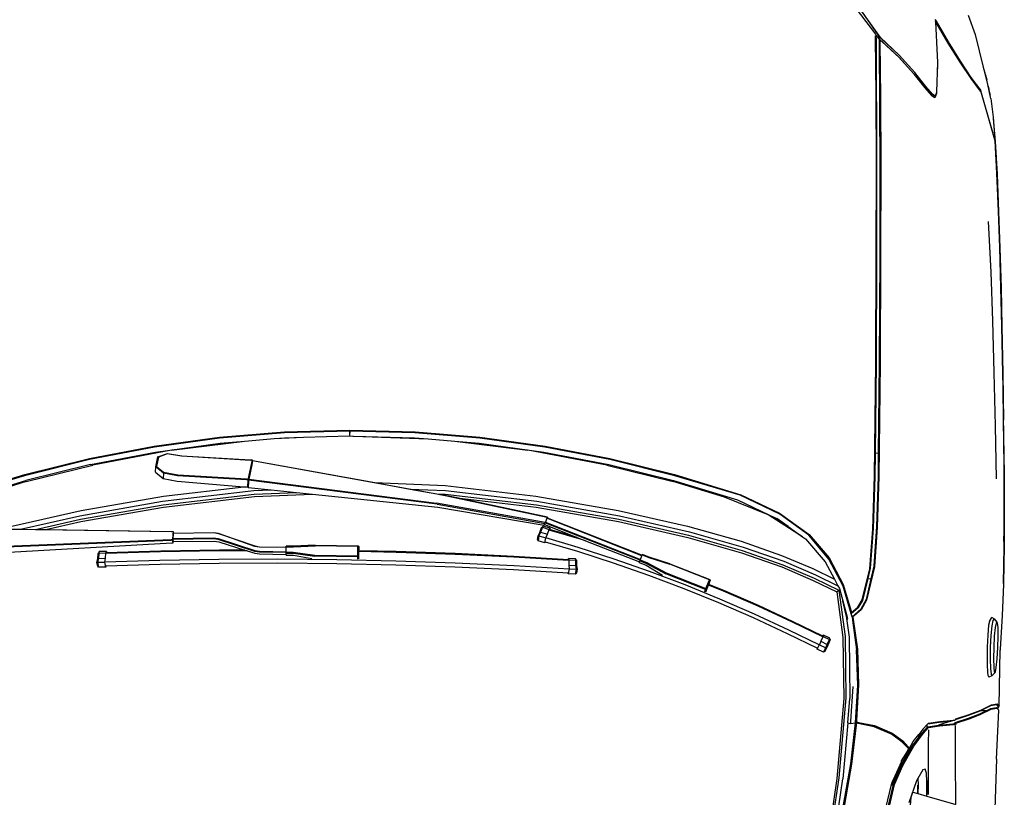
# Model space of a CAD drawing. Units: inches. Extents: x 1319 to 2030, y 219 to 1069.
# Tile 14 of 28: x 1444 to 1498, y 473 to 515. Entities that reach past the tile are written whole.
import ezdxf

# ---------------------------------------------------------------- set-up
doc = ezdxf.new("R2010")
doc.units = ezdxf.units.IN
doc.header["$MEASUREMENT"] = 0
doc.layers.get('0').update_dxf_attribs({"color": 12})
doc.layers.add('C-PRKG-VEHC', color=8, linetype='Continuous', lineweight=13)
doc.layers.add('Edges', color=250, linetype='Continuous')

# ---------------------------------------------------------------- blocks, each defined once
blk = doc.blocks.new('Nissan Qashqai pl')
at = {"layer": 'Edges'}
for p, q in [((8.1902, 12.8233), (8.2543, 12.8243)), ((8.2543, 12.8243), (8.2094, 12.8235)), ((8.2543, 12.8243), (8.2094, 12.8235)), ((8.2544, 12.8242), (8.2094, 12.8235)), ((8.2693, 12.8245), (8.2543, 12.8243)), ((8.3166, 12.8249), (8.2544, 12.8242)), ((8.3098, 12.825), (8.2693, 12.8245)), ((8.3159, 12.825), (8.2693, 12.8245)), ((8.3159, 12.825), (8.3098, 12.825)), ((8.3159, 12.825), (8.3163, 12.825)), ((8.3163, 12.825), (8.3657, 12.8252)), ((8.3163, 12.825), (8.3597, 12.8252)), ((8.3764, 12.8251), (8.3166, 12.8249)), ((8.3597, 12.8252), (8.3657, 12.8252)), ((8.3657, 12.8252), (8.3663, 12.8252)), ((8.3663, 12.8252), (8.3747, 12.8252)), ((8.3764, 12.8251), (8.3663, 12.8252)), ((8.3747, 12.8252), (8.3757, 12.8252)), ((8.3757, 12.8252), (8.4282, 12.8249)), ((8.4069, 12.8249), (8.3764, 12.8251)), ((8.4219, 12.8246), (8.4069, 12.8249)), ((8.4292, 12.8248), (8.4069, 12.8249)), ((8.4282, 12.8249), (8.4799, 12.8239)), ((8.4799, 12.8239), (8.4292, 12.8248)), ((8.4799, 12.8239), (8.4811, 12.8239)), ((8.4811, 12.8239), (8.5241, 12.8222)), ((7.8676, 12.8123), (7.7998, 12.7928)), ((7.8012, 12.7929), (7.8681, 12.8121)), ((7.8363, 12.8097), (7.8676, 12.8123)), ((7.8381, 12.81), (7.87, 12.8126)), ((7.8676, 12.8123), (7.8681, 12.8121)), ((7.869, 12.8124), (7.8681, 12.8121)), ((7.9137, 12.815), (7.869, 12.8124)), ((7.87, 12.8126), (7.9151, 12.8152)), ((7.9658, 12.8172), (7.9137, 12.815)), ((7.9151, 12.8152), (7.9668, 12.8174)), ((8.016, 12.8189), (7.9658, 12.8172)), ((7.9668, 12.8174), (8.0168, 12.8191)), ((8.0713, 12.8205), (8.016, 12.8189)), ((8.0168, 12.8191), (8.0718, 12.8207)), ((8.1249, 12.8218), (8.0713, 12.8205)), ((8.0718, 12.8207), (8.1251, 12.822)), ((8.1176, 12.8087), (8.1888, 12.8107)), ((8.1901, 12.8232), (8.1249, 12.8218)), ((8.1251, 12.822), (8.1902, 12.8233)), ((8.1888, 12.8107), (8.2622, 12.8125)), ((8.2094, 12.8235), (8.1901, 12.8232)), ((8.2622, 12.8125), (8.3356, 12.8141)), ((8.5241, 12.8222), (8.5707, 12.8193)), ((8.5287, 12.8112), (8.5269, 12.8082)), ((8.5287, 12.8112), (8.5331, 12.815)), ((8.5287, 12.8112), (8.531, 12.8095)), ((8.5347, 12.8159), (8.5331, 12.815)), ((8.5331, 12.815), (8.5346, 12.8138)), ((8.5346, 12.8138), (8.5406, 12.8125)), ((8.5407, 12.8167), (8.5347, 12.8159)), ((8.5406, 12.8125), (8.5526, 12.8114)), ((8.5527, 12.8169), (8.5407, 12.8167)), ((8.5526, 12.8114), (8.5681, 12.8107)), ((8.5682, 12.8164), (8.5527, 12.8169)), ((8.5681, 12.8107), (8.5836, 12.8104)), ((8.5837, 12.8154), (8.5682, 12.8164)), ((8.5707, 12.8193), (8.5719, 12.8193)), ((8.6489, 12.8179), (8.5719, 12.8193)), ((8.5836, 12.8104), (8.5957, 12.8107)), ((8.5958, 12.8141), (8.5837, 12.8154)), ((8.5957, 12.8107), (8.6017, 12.8114)), ((8.6018, 12.8129), (8.5958, 12.8141)), ((8.6017, 12.8114), (8.6032, 12.8121)), ((8.6032, 12.8121), (8.6018, 12.8129)), ((8.6073, 12.808), (8.6032, 12.8121)), ((8.646, 12.8153), (8.6489, 12.8179)), ((8.646, 12.8153), (8.646, 12.8153)), ((8.6472, 12.8076), (8.646, 12.8153)), ((8.647, 12.8142), (8.6498, 12.8168)), ((8.6482, 12.8067), (8.647, 12.8142)), ((8.6489, 12.8179), (8.6527, 12.8156)), ((8.6498, 12.8168), (8.6524, 12.8153)), ((8.651, 12.814), (8.652, 12.815)), ((8.6524, 12.8064), (8.651, 12.814)), ((8.652, 12.815), (8.6524, 12.8153)), ((8.6534, 12.8073), (8.652, 12.815)), ((8.6524, 12.8153), (8.6527, 12.8156)), ((8.6527, 12.8156), (8.6537, 12.8167)), ((8.6547, 12.8176), (8.6537, 12.8167)), ((8.6537, 12.8167), (8.6537, 12.8166)), ((8.7222, 12.8144), (8.6547, 12.8176)), ((8.7222, 12.8144), (8.7908, 12.812)), ((7.7673, 12.7961), (7.8058, 12.8055)), ((7.7673, 12.7961), (7.7848, 12.8012)), ((7.7835, 12.8007), (7.7835, 12.8007)), ((7.8087, 12.8062), (7.7848, 12.8012)), ((7.7865, 12.8013), (7.7866, 12.8013)), ((7.7936, 12.8029), (7.7977, 12.8038)), ((7.8106, 12.8065), (7.8087, 12.8062)), ((7.8106, 12.8065), (7.8107, 12.8065)), ((7.8107, 12.8065), (7.8363, 12.8097)), ((7.8363, 12.8097), (7.8381, 12.81)), ((7.9803, 12.803), (8.05, 12.8066)), ((8.05, 12.8066), (8.1176, 12.8087)), ((8.5322, 12.8047), (8.5269, 12.8082)), ((8.531, 12.8095), (8.5385, 12.8079)), ((8.5322, 12.8047), (8.5375, 12.8036)), ((8.5375, 12.8036), (8.5513, 12.8023)), ((8.5385, 12.8079), (8.5518, 12.8066)), ((8.5513, 12.8023), (8.5678, 12.8016)), ((8.5518, 12.8066), (8.568, 12.8059)), ((8.5678, 12.8016), (8.5844, 12.8014)), ((8.568, 12.8059), (8.5842, 12.8057)), ((8.5842, 12.8057), (8.5974, 12.8061)), ((8.5844, 12.8014), (8.5921, 12.8016)), ((8.5921, 12.8016), (8.6021, 12.8022)), ((8.5974, 12.8061), (8.6049, 12.8069)), ((8.6021, 12.8022), (8.6065, 12.8027)), ((8.6049, 12.8069), (8.6073, 12.808)), ((8.6065, 12.8027), (8.6093, 12.804)), ((8.6073, 12.808), (8.6093, 12.804)), ((8.6546, 12.7926), (8.6472, 12.8076)), ((8.655, 12.7929), (8.6482, 12.8067)), ((8.655, 12.801), (8.6524, 12.8064)), ((8.6608, 12.7921), (8.6534, 12.8073)), ((8.6598, 12.7913), (8.655, 12.801)), ((8.655, 12.7929), (8.655, 12.801)), ((7.6953, 12.7753), (7.7223, 12.7851)), ((7.7223, 12.7851), (7.7673, 12.7961)), ((7.7814, 12.7791), (7.7991, 12.7923)), ((7.7984, 12.7909), (7.7828, 12.7793)), ((7.7976, 12.792), (7.7991, 12.7923)), ((7.8007, 12.7926), (7.7984, 12.7909)), ((7.7991, 12.7923), (7.7998, 12.7928)), ((7.7995, 12.7924), (7.8007, 12.7926)), ((7.8012, 12.7929), (7.8007, 12.7926)), ((8.6606, 12.7768), (8.6546, 12.7926)), ((8.6556, 12.7918), (8.655, 12.7929)), ((8.655, 12.7922), (8.655, 12.7929)), ((8.6616, 12.7758), (8.6556, 12.7918)), ((8.6657, 12.7758), (8.6598, 12.7913)), ((8.6667, 12.7767), (8.6608, 12.7921)), ((7.7591, 12.7641), (7.7814, 12.7791)), ((7.7828, 12.7793), (7.7606, 12.7644)), ((8.6667, 12.7584), (8.6606, 12.7768)), ((8.6675, 12.758), (8.6616, 12.7758)), ((8.6718, 12.7574), (8.6657, 12.7758)), ((8.6728, 12.7584), (8.6667, 12.7767)), ((7.7325, 12.7476), (7.7591, 12.7641)), ((7.7606, 12.7644), (7.7341, 12.7478)), ((8.6675, 12.758), (8.6667, 12.7584)), ((8.6679, 12.7578), (8.6675, 12.758)), ((8.6676, 12.7576), (8.6675, 12.7576)), ((8.6675, 12.7576), (8.6675, 12.7576)), ((8.6675, 12.7576), (8.6676, 12.7576)), ((8.6676, 12.7576), (8.6677, 12.7576)), ((8.6677, 12.7576), (8.6677, 12.7576)), ((8.6677, 12.7576), (8.6682, 12.7576)), ((8.6682, 12.7576), (8.6679, 12.7578)), ((8.6682, 12.7576), (8.6692, 12.7566)), ((8.6682, 12.7572), (8.6682, 12.7576)), ((8.6684, 12.7554), (8.6682, 12.7572)), ((8.6682, 12.7572), (8.6692, 12.7566)), ((8.6692, 12.7566), (8.6697, 12.7519)), ((8.6729, 12.7568), (8.6718, 12.7574)), ((8.674, 12.7578), (8.6728, 12.7584)), ((8.6733, 12.7566), (8.6729, 12.7568)), ((8.6735, 12.7544), (8.6733, 12.7566)), ((8.6742, 12.7576), (8.674, 12.7578)), ((8.6742, 12.7584), (8.6743, 12.7582)), ((8.6744, 12.755), (8.6742, 12.7576)), ((8.6744, 12.7576), (8.6742, 12.7576)), ((8.6744, 12.7578), (8.6744, 12.7576)), ((8.6773, 12.7577), (8.6744, 12.7576)), ((8.6791, 12.7578), (8.677, 12.7578)), ((8.6791, 12.7577), (8.6773, 12.7577)), ((8.7205, 12.7579), (8.6791, 12.7578)), ((8.6791, 12.7577), (8.6791, 12.7578)), ((8.6878, 12.7577), (8.6791, 12.7578)), ((8.6878, 12.7577), (8.6791, 12.7577)), ((8.6878, 12.7577), (8.6878, 12.7577)), ((8.6911, 12.7577), (8.6878, 12.7577)), ((8.7205, 12.7579), (8.6911, 12.7577)), ((8.7849, 12.7582), (8.7205, 12.7579)), ((8.7734, 12.7181), (8.7849, 12.7582)), ((7.7038, 12.731), (7.7325, 12.7476)), ((7.7341, 12.7478), (7.7056, 12.7314)), ((8.6684, 12.7554), (8.6685, 12.7549)), ((8.6684, 12.755), (8.6684, 12.7554)), ((8.6703, 12.7361), (8.6684, 12.755)), ((8.6697, 12.7519), (8.6698, 12.7516)), ((8.6714, 12.7353), (8.6697, 12.7519)), ((8.6698, 12.7516), (8.6755, 12.7343)), ((8.6754, 12.7353), (8.6735, 12.7544)), ((8.6764, 12.736), (8.6744, 12.755)), ((7.701, 12.73), (7.7024, 12.7301)), ((7.7024, 12.7301), (7.7038, 12.731)), ((7.7024, 12.7301), (7.7034, 12.7301)), ((7.7056, 12.7314), (7.7034, 12.7301)), ((7.7034, 12.7301), (7.7048, 12.7302)), ((7.7048, 12.7302), (7.7608, 12.7329)), ((7.7058, 12.7308), (7.7048, 12.7302)), ((7.7608, 12.7329), (7.8014, 12.7318)), ((7.7688, 12.7328), (7.7688, 12.734)), ((7.8014, 12.7318), (7.8022, 12.7316)), ((7.8022, 12.7316), (7.8037, 12.7315)), ((7.8022, 12.7316), (7.8072, 12.73)), ((7.8037, 12.7315), (7.8096, 12.7294)), ((7.8072, 12.73), (7.8045, 12.7263)), ((7.8096, 12.7294), (7.8066, 12.7254)), ((7.8072, 12.73), (7.8087, 12.7283)), ((8.6727, 12.7207), (8.6703, 12.7361)), ((8.6737, 12.7197), (8.6714, 12.7353)), ((8.6755, 12.7343), (8.6754, 12.7353)), ((8.6777, 12.7196), (8.6755, 12.7343)), ((8.6764, 12.7359), (8.6764, 12.736)), ((8.6788, 12.7205), (8.6764, 12.7359)), ((7.7938, 12.7171), (7.7748, 12.7018)), ((7.7959, 12.7161), (7.7772, 12.7011)), ((7.8045, 12.7263), (7.7938, 12.7171)), ((7.8062, 12.725), (7.7959, 12.7161)), ((7.8062, 12.725), (7.8087, 12.7283)), ((7.8066, 12.7254), (7.8062, 12.725)), ((8.6737, 12.7197), (8.6727, 12.7207)), ((8.6746, 12.7189), (8.6737, 12.7197)), ((8.6785, 12.7189), (8.6746, 12.7189)), ((8.6805, 12.7132), (8.6746, 12.7189)), ((8.6785, 12.7189), (8.6777, 12.7196)), ((8.6815, 12.7162), (8.6785, 12.7189)), ((8.687, 12.7132), (8.6788, 12.7205)), ((8.6815, 12.7162), (8.6818, 12.7154)), ((8.6817, 12.716), (8.6815, 12.7162)), ((8.6817, 12.716), (8.6818, 12.7154)), ((8.6859, 12.7122), (8.6817, 12.716)), ((8.6818, 12.7204), (8.7012, 12.7203)), ((8.6818, 12.7154), (8.6902, 12.7081)), ((8.7012, 12.7203), (8.7012, 12.7203)), ((8.7012, 12.7203), (8.7026, 12.7203)), ((8.7026, 12.7203), (8.7026, 12.7203)), ((8.7026, 12.7203), (8.7072, 12.7203)), ((8.7072, 12.7203), (8.7072, 12.7203)), ((8.7072, 12.7203), (8.7273, 12.7202)), ((8.7273, 12.7202), (8.7273, 12.7201)), ((8.7273, 12.7202), (8.7354, 12.7202)), ((8.7354, 12.7201), (8.7354, 12.7202)), ((8.7354, 12.7202), (8.742, 12.7202)), ((8.7415, 12.7177), (8.7361, 12.7158)), ((8.7361, 12.7158), (8.7373, 12.7128)), ((8.7534, 12.7185), (8.7415, 12.7177)), ((8.742, 12.7201), (8.742, 12.7202)), ((8.742, 12.7202), (8.742, 12.7201)), ((8.742, 12.7202), (8.742, 12.7202)), ((8.742, 12.7202), (8.7426, 12.7202)), ((8.7426, 12.7201), (8.7426, 12.7202)), ((8.7426, 12.7202), (8.7433, 12.7202)), ((8.7433, 12.7201), (8.7433, 12.7202)), ((8.7433, 12.7202), (8.7711, 12.7201)), ((8.7711, 12.7201), (8.7516, 12.72)), ((8.7718, 12.7181), (8.7534, 12.7185)), ((8.7698, 12.7058), (8.7734, 12.7181)), ((8.7734, 12.7181), (8.7718, 12.7181)), ((7.7748, 12.7018), (7.7507, 12.6803)), ((8.6805, 12.7132), (8.6884, 12.7071)), ((8.6927, 12.7071), (8.6859, 12.7122)), ((8.7042, 12.7002), (8.687, 12.7132)), ((8.6917, 12.7071), (8.6884, 12.7071)), ((8.698, 12.6996), (8.6884, 12.7071)), ((8.6902, 12.7081), (8.6917, 12.7071)), ((8.6917, 12.7071), (8.7075, 12.6955)), ((8.6927, 12.7071), (8.6923, 12.7071)), ((8.7032, 12.6992), (8.6927, 12.7071)), ((8.7373, 12.7128), (8.7492, 12.7059)), ((8.7492, 12.7059), (8.7572, 12.7062)), ((8.7492, 12.7059), (8.7524, 12.704)), ((8.7524, 12.704), (8.7828, 12.6934)), ((8.7572, 12.7062), (8.7698, 12.7058)), ((8.7698, 12.7057), (8.7583, 12.706)), ((8.7678, 12.6988), (8.7698, 12.7057)), ((8.7698, 12.7057), (8.7698, 12.7058)), ((7.753, 12.6794), (7.776, 12.6999)), ((7.776, 12.6999), (7.7539, 12.68)), ((7.7772, 12.7011), (7.776, 12.6999)), ((8.697, 12.685), (8.7055, 12.6927)), ((8.6979, 12.6839), (8.7062, 12.6915)), ((8.7071, 12.6942), (8.698, 12.6996)), ((8.7062, 12.6915), (8.6987, 12.6845)), ((8.7302, 12.684), (8.7032, 12.6992)), ((8.7312, 12.6851), (8.7042, 12.7002)), ((8.7055, 12.6927), (8.7071, 12.6942)), ((8.7062, 12.6915), (8.7067, 12.6919)), ((8.7067, 12.6919), (8.7083, 12.6934)), ((8.7071, 12.6942), (8.7083, 12.6934)), ((8.7075, 12.6955), (8.7346, 12.6806)), ((8.7083, 12.6934), (8.7083, 12.6934)), ((8.7083, 12.6934), (8.7083, 12.6934)), ((8.7102, 12.6923), (8.7083, 12.6934)), ((8.7083, 12.6934), (8.7083, 12.6934)), ((8.7108, 12.6919), (8.7102, 12.6923)), ((8.7102, 12.6923), (8.7102, 12.6923)), ((8.7257, 12.6833), (8.7108, 12.6919)), ((8.7248, 12.6836), (8.7108, 12.6919)), ((8.7748, 12.6967), (8.7678, 12.6988)), ((8.7916, 12.6954), (8.7748, 12.6967)), ((7.7261, 12.6543), (7.7507, 12.6803)), ((7.753, 12.6794), (7.7281, 12.6524)), ((7.7507, 12.6803), (7.7286, 12.6561)), ((7.7539, 12.68), (7.7324, 12.6565)), ((8.6864, 12.6706), (8.697, 12.685)), ((8.6875, 12.6698), (8.6979, 12.6839)), ((8.6924, 12.676), (8.6883, 12.6704)), ((8.6987, 12.6845), (8.6924, 12.676)), ((8.6924, 12.676), (8.6924, 12.6762)), ((8.7257, 12.6833), (8.7248, 12.6836)), ((8.7257, 12.6832), (8.7257, 12.6833)), ((8.7257, 12.6832), (8.7508, 12.672)), ((8.7529, 12.6741), (8.7302, 12.684)), ((8.7574, 12.6737), (8.7312, 12.6851)), ((8.7346, 12.6806), (8.7491, 12.6738)), ((8.7346, 12.6806), (8.7577, 12.6709)), ((8.6759, 12.6459), (8.6864, 12.6706)), ((8.6772, 12.6454), (8.6875, 12.6698)), ((8.6883, 12.6704), (8.6777, 12.6457)), ((8.7508, 12.672), (8.7491, 12.6738)), ((8.7491, 12.6738), (8.7576, 12.6699)), ((8.7532, 12.6708), (8.7508, 12.672)), ((8.7529, 12.6741), (8.7577, 12.6709)), ((8.757, 12.6724), (8.7529, 12.6741)), ((8.7575, 12.6698), (8.7532, 12.6708)), ((8.7587, 12.672), (8.757, 12.6724)), ((8.7931, 12.6653), (8.7574, 12.6737)), ((8.7576, 12.6699), (8.7575, 12.6698)), ((8.7881, 12.6621), (8.7575, 12.6698)), ((8.7582, 12.6707), (8.7576, 12.6699)), ((8.7577, 12.6709), (8.7582, 12.6707)), ((8.759, 12.6717), (8.7582, 12.6707)), ((8.7587, 12.672), (8.759, 12.6717)), ((8.7591, 12.6719), (8.7587, 12.672)), ((8.7591, 12.6719), (8.759, 12.6717)), ((8.7925, 12.664), (8.7591, 12.6719)), ((7.7261, 12.6543), (7.6762, 12.6186)), ((7.6762, 12.6186), (7.7233, 12.6514)), ((7.6771, 12.6135), (7.7215, 12.6473)), ((7.7215, 12.6473), (7.7221, 12.6478)), ((7.7232, 12.6486), (7.7221, 12.6478)), ((7.7281, 12.6524), (7.7232, 12.6486)), ((7.7245, 12.6486), (7.7232, 12.6486)), ((7.7267, 12.6539), (7.7233, 12.6514)), ((7.7261, 12.6476), (7.7238, 12.6476)), ((7.7294, 12.6487), (7.7245, 12.6486)), ((7.7279, 12.6477), (7.7261, 12.6476)), ((7.7286, 12.6561), (7.7267, 12.6539)), ((7.8048, 12.6483), (7.7279, 12.6477)), ((7.7299, 12.6537), (7.7281, 12.6524)), ((7.7281, 12.6524), (7.7349, 12.6524)), ((7.731, 12.6487), (7.7294, 12.6487)), ((7.7324, 12.6565), (7.7299, 12.6537)), ((7.7299, 12.6537), (7.7334, 12.6537)), ((7.764, 12.6489), (7.731, 12.6487)), ((7.7334, 12.6537), (7.8083, 12.6544)), ((7.7349, 12.6524), (7.768, 12.6527)), ((7.7662, 12.6489), (7.764, 12.6489)), ((7.7811, 12.649), (7.7662, 12.6489)), ((7.768, 12.6527), (7.7692, 12.6527)), ((7.7692, 12.6527), (7.7844, 12.6528)), ((7.7822, 12.649), (7.7811, 12.649)), ((7.8057, 12.6491), (7.7822, 12.649)), ((7.7844, 12.6528), (7.8078, 12.653)), ((7.9014, 12.6487), (7.8048, 12.6483)), ((7.8233, 12.6492), (7.8057, 12.6491)), ((7.8078, 12.653), (7.8233, 12.6531)), ((7.8083, 12.6544), (7.904, 12.6547)), ((7.8233, 12.6531), (7.9036, 12.6534)), ((7.902, 12.6495), (7.8233, 12.6492)), ((8.0273, 12.6485), (7.9014, 12.6487)), ((8.0275, 12.6493), (7.902, 12.6495)), ((7.9036, 12.6534), (8.0275, 12.6533)), ((7.904, 12.6547), (8.0276, 12.6545)), ((8.1753, 12.6479), (8.0273, 12.6485)), ((8.0275, 12.6533), (8.1755, 12.6527)), ((8.1754, 12.6487), (8.0275, 12.6493)), ((8.0276, 12.6545), (8.1753, 12.6539)), ((8.1753, 12.6539), (8.3324, 12.6521)), ((8.3318, 12.6462), (8.1753, 12.6479)), ((8.3002, 12.6474), (8.1754, 12.6487)), ((8.1755, 12.6527), (8.3005, 12.6514)), ((8.3005, 12.6514), (8.3002, 12.6474)), ((8.332, 12.6471), (8.3002, 12.6474)), ((8.3005, 12.6514), (8.3324, 12.651)), ((8.4042, 12.6447), (8.332, 12.6471)), ((8.3324, 12.6521), (8.4022, 12.6498)), ((8.3324, 12.651), (8.4014, 12.6488)), ((8.4014, 12.6488), (8.4559, 12.6451)), ((8.4022, 12.6498), (8.4571, 12.6459)), ((8.4049, 12.6437), (8.3318, 12.6462)), ((8.4588, 12.6405), (8.4042, 12.6447)), ((8.4595, 12.6395), (8.4049, 12.6437)), ((8.4559, 12.6451), (8.4736, 12.6409)), ((8.4571, 12.6459), (8.5029, 12.635)), ((8.4729, 12.6372), (8.4588, 12.6405)), ((8.5025, 12.6293), (8.4595, 12.6395)), ((8.4729, 12.6372), (8.4736, 12.6409)), ((8.5032, 12.6301), (8.4729, 12.6372)), ((8.4736, 12.6409), (8.5018, 12.6344)), ((8.5018, 12.6344), (8.5155, 12.6274)), ((8.5029, 12.635), (8.5163, 12.6279)), ((8.6716, 12.6242), (8.6759, 12.6459)), ((8.6772, 12.6454), (8.6721, 12.6201)), ((8.6777, 12.6457), (8.6727, 12.6213)), ((8.5125, 12.6231), (8.5025, 12.6293)), ((8.5132, 12.624), (8.5032, 12.6301)), ((8.5177, 12.617), (8.5125, 12.6231)), ((8.5132, 12.624), (8.5216, 12.6139)), ((8.5155, 12.6274), (8.5258, 12.6151)), ((8.5163, 12.6279), (8.5237, 12.6189)), ((8.5294, 12.6167), (8.5706, 12.6226)), ((8.5304, 12.6157), (8.5715, 12.6215)), ((8.5706, 12.6226), (8.6197, 12.6241)), ((8.6203, 12.6229), (8.5715, 12.6215)), ((8.6197, 12.6241), (8.6683, 12.6215)), ((8.6203, 12.6229), (8.6204, 12.6229)), ((8.6721, 12.6201), (8.6204, 12.6229)), ((8.6683, 12.6215), (8.671, 12.6214)), ((8.671, 12.6214), (8.6716, 12.6242)), ((8.671, 12.6214), (8.6721, 12.6201)), ((8.6727, 12.6213), (8.6721, 12.6201)), ((8.6733, 12.6129), (8.6721, 12.6201)), ((8.7287, 12.6134), (8.6721, 12.6201)), ((8.6727, 12.6213), (8.6753, 12.621)), ((8.6753, 12.621), (8.7292, 12.6146)), ((8.4814, 12.6029), (8.5166, 12.6135)), ((8.5216, 12.6139), (8.4838, 12.6027)), ((8.5039, 12.6023), (8.528, 12.6088)), ((8.5216, 12.6068), (8.5039, 12.6023)), ((8.5166, 12.6135), (8.5197, 12.6145)), ((8.5197, 12.6145), (8.5177, 12.617)), ((8.5197, 12.6145), (8.5216, 12.6139)), ((8.5258, 12.6151), (8.5216, 12.6139)), ((8.5216, 12.6068), (8.5538, 12.6111)), ((8.5301, 12.609), (8.5216, 12.6068)), ((8.5237, 12.6189), (8.5259, 12.6162)), ((8.5259, 12.6162), (8.5258, 12.6151)), ((8.5258, 12.6151), (8.5304, 12.6157)), ((8.5259, 12.6162), (8.5294, 12.6167)), ((8.5304, 12.6157), (8.5304, 12.6157)), ((8.5531, 12.6055), (8.6375, 12.6066)), ((8.5538, 12.6111), (8.6387, 12.6123)), ((8.622, 12.6161), (8.6699, 12.6132)), ((8.6375, 12.6066), (8.7481, 12.5968)), ((8.6721, 12.6093), (8.6387, 12.6123)), ((8.6699, 12.6132), (8.6721, 12.613)), ((8.6721, 12.6127), (8.6721, 12.613)), ((8.6721, 12.613), (8.6733, 12.6129)), ((8.6721, 12.6093), (8.6733, 12.6129)), ((8.6721, 12.6093), (8.7496, 12.6025)), ((8.8666, 12.5888), (8.7287, 12.6134)), ((8.7292, 12.6146), (8.8666, 12.5901)), ((8.4444, 12.5834), (8.4814, 12.6029)), ((8.4838, 12.6027), (8.4462, 12.5833)), ((8.468, 12.5648), (8.4831, 12.5957)), ((8.4725, 12.563), (8.4889, 12.5969)), ((8.4737, 12.5908), (8.4831, 12.5957)), ((8.4756, 12.5615), (8.4914, 12.5942)), ((8.4831, 12.5957), (8.4867, 12.5977)), ((8.4867, 12.5977), (8.5039, 12.6023)), ((8.4889, 12.5969), (8.5531, 12.6055)), ((8.4914, 12.5942), (8.4889, 12.5969)), ((8.4914, 12.5942), (8.5544, 12.6026)), ((8.5544, 12.6026), (8.6386, 12.6037)), ((8.6386, 12.6037), (8.7491, 12.594)), ((8.7481, 12.5968), (8.8745, 12.5782)), ((8.7491, 12.594), (8.8754, 12.5755)), ((8.8761, 12.5839), (8.7496, 12.6025)), ((8.4122, 12.5558), (8.4444, 12.5834)), ((8.4462, 12.5833), (8.4134, 12.5554)), ((8.4499, 12.5782), (8.4737, 12.5908)), ((8.4594, 12.5611), (8.4737, 12.5908)), ((8.5554, 12.5847), (8.551, 12.5757)), ((8.5529, 12.5751), (8.5572, 12.5841)), ((8.5574, 12.5849), (8.5554, 12.5847)), ((8.5572, 12.5841), (8.5554, 12.5847)), ((8.5639, 12.581), (8.5572, 12.5841)), ((8.5574, 12.5849), (8.5584, 12.5846)), ((8.5582, 12.5845), (8.5574, 12.5849)), ((8.5584, 12.5846), (8.5649, 12.5816)), ((8.5595, 12.572), (8.5639, 12.581)), ((8.5687, 12.5791), (8.5639, 12.581)), ((8.5644, 12.5701), (8.5687, 12.5791)), ((8.5649, 12.5816), (8.5693, 12.5799)), ((8.5687, 12.5791), (8.5693, 12.5799)), ((8.5749, 12.5757), (8.5687, 12.5791)), ((8.5693, 12.5799), (8.5739, 12.5774)), ((8.4183, 12.5508), (8.4499, 12.5782)), ((8.5527, 12.5749), (8.5323, 12.5332)), ((8.5537, 12.5747), (8.5332, 12.5329)), ((8.5647, 12.57), (8.5441, 12.5279)), ((8.5487, 12.5256), (8.5692, 12.5674)), ((8.5527, 12.5749), (8.551, 12.5757)), ((8.551, 12.5757), (8.5528, 12.5751)), ((8.5528, 12.5751), (8.5527, 12.5749)), ((8.5528, 12.5751), (8.5529, 12.5751)), ((8.5529, 12.5751), (8.5537, 12.5747)), ((8.5537, 12.5747), (8.5595, 12.572)), ((8.5595, 12.572), (8.5644, 12.5701)), ((8.5644, 12.5701), (8.5647, 12.57)), ((8.5647, 12.57), (8.5692, 12.5675)), ((8.5692, 12.5674), (8.5692, 12.5675)), ((8.5692, 12.5675), (8.5705, 12.5668)), ((8.5705, 12.5668), (8.5692, 12.5674)), ((8.5749, 12.5757), (8.5705, 12.5668)), ((8.5739, 12.5774), (8.5749, 12.5757)), ((8.3826, 12.5151), (8.4122, 12.5558)), ((8.4134, 12.5554), (8.3844, 12.5157)), ((8.4411, 12.5178), (8.4594, 12.5611)), ((8.4493, 12.5212), (8.468, 12.5648)), ((8.454, 12.5196), (8.4725, 12.563)), ((8.4571, 12.5184), (8.4756, 12.5615)), ((8.4154, 12.5468), (8.3852, 12.4994)), ((8.3901, 12.5113), (8.4154, 12.5468)), ((8.4011, 12.5269), (8.4154, 12.5468)), ((8.4156, 12.547), (8.4154, 12.5468)), ((8.4156, 12.547), (8.4183, 12.5508)), ((8.4011, 12.5269), (8.3901, 12.5113)), ((8.3904, 12.512), (8.4011, 12.5269)), ((8.5323, 12.5332), (8.5103, 12.4859)), ((8.5332, 12.5329), (8.5112, 12.4856)), ((8.5441, 12.5279), (8.5222, 12.4807)), ((8.5269, 12.4785), (8.5487, 12.5256)), ((8.3573, 12.4618), (8.3826, 12.5151)), ((8.3844, 12.5157), (8.3582, 12.4606)), ((8.39, 12.5111), (8.3901, 12.5113)), ((8.3901, 12.5113), (8.3904, 12.512)), ((8.4217, 12.4622), (8.4411, 12.5178)), ((8.4296, 12.4651), (8.4493, 12.5212)), ((8.4343, 12.4637), (8.454, 12.5196)), ((8.4375, 12.4627), (8.4571, 12.5184)), ((8.3852, 12.4994), (8.3608, 12.4393)), ((8.3646, 12.4572), (8.39, 12.5111)), ((8.3648, 12.4579), (8.39, 12.5111)), ((8.39, 12.5111), (8.3852, 12.4994)), ((8.5103, 12.4859), (8.4895, 12.4381)), ((8.5112, 12.4856), (8.4904, 12.4377)), ((8.5222, 12.4807), (8.5014, 12.4329)), ((8.5062, 12.431), (8.5269, 12.4785)), ((8.3296, 12.3703), (8.3573, 12.4618)), ((8.3582, 12.4606), (8.3311, 12.3708)), ((8.3377, 12.3689), (8.3646, 12.4572)), ((8.3646, 12.4572), (8.3648, 12.4579)), ((8.3648, 12.4579), (8.3648, 12.4579)), ((8.4009, 12.3883), (8.4217, 12.4622)), ((8.4084, 12.3907), (8.4296, 12.4651)), ((8.4133, 12.3896), (8.4343, 12.4637)), ((8.4165, 12.3888), (8.4375, 12.4627)), ((8.3608, 12.4393), (8.3392, 12.3684)), ((8.3608, 12.4393), (8.3608, 12.4393)), ((8.4895, 12.4381), (8.4811, 12.4174)), ((8.5014, 12.4329), (8.4817, 12.3847)), ((8.4904, 12.4377), (8.482, 12.4171)), ((8.4866, 12.3829), (8.5062, 12.431)), ((8.4526, 12.3639), (8.4742, 12.4188)), ((8.4747, 12.4185), (8.4532, 12.3636)), ((8.4742, 12.4188), (8.4754, 12.4193)), ((8.4747, 12.4185), (8.4742, 12.4188)), ((8.4754, 12.4193), (8.4747, 12.4185)), ((8.4869, 12.4136), (8.4747, 12.4185)), ((8.4754, 12.4193), (8.4876, 12.4144)), ((8.4791, 12.4183), (8.4754, 12.4193)), ((8.4811, 12.4174), (8.4791, 12.4183)), ((8.482, 12.4171), (8.4811, 12.4174)), ((8.4912, 12.4133), (8.482, 12.4171)), ((8.4654, 12.3587), (8.4869, 12.4136)), ((8.4881, 12.4131), (8.4666, 12.3582)), ((8.4869, 12.4136), (8.4876, 12.4144)), ((8.4881, 12.4131), (8.4869, 12.4136)), ((8.4876, 12.4144), (8.4912, 12.4133)), ((8.4876, 12.4144), (8.4881, 12.4131)), ((8.4914, 12.4121), (8.4881, 12.4131)), ((8.4913, 12.4133), (8.4912, 12.4133)), ((8.4913, 12.4132), (8.4913, 12.4133)), ((8.3864, 12.2945), (8.4084, 12.3907)), ((8.3913, 12.2935), (8.4133, 12.3896)), ((8.3792, 12.2926), (8.4009, 12.3883)), ((8.3945, 12.2929), (8.4165, 12.3888)), ((8.4817, 12.3847), (8.4633, 12.3359)), ((8.4683, 12.3345), (8.4866, 12.3829)), ((8.3076, 12.281), (8.3296, 12.3703)), ((8.3311, 12.3708), (8.3089, 12.2811)), ((8.3157, 12.2795), (8.3377, 12.3689)), ((8.3166, 12.2767), (8.3392, 12.3684)), ((8.4526, 12.3639), (8.4434, 12.3353)), ((8.4439, 12.335), (8.4532, 12.3636)), ((8.4509, 12.3322), (8.4654, 12.3587)), ((8.4521, 12.3317), (8.4666, 12.3582)), ((8.4547, 12.3309), (8.4682, 12.3538)), ((8.4434, 12.3353), (8.4397, 12.326)), ((8.4403, 12.3257), (8.4439, 12.335)), ((8.4633, 12.3359), (8.4461, 12.2868)), ((8.3894, 12.1944), (8.4409, 12.3255)), ((8.4415, 12.3252), (8.3899, 12.1941)), ((8.3951, 12.192), (8.4467, 12.3231)), ((8.4479, 12.3226), (8.3963, 12.1915)), ((8.4209, 12.2475), (8.4502, 12.3219)), ((8.4403, 12.3257), (8.4397, 12.326)), ((8.4409, 12.3255), (8.4403, 12.3257)), ((8.4415, 12.3252), (8.4409, 12.3255)), ((8.4467, 12.3231), (8.4415, 12.3252)), ((8.4472, 12.3229), (8.4467, 12.3231)), ((8.4472, 12.3229), (8.4509, 12.3322)), ((8.4479, 12.3226), (8.4472, 12.3229)), ((8.4484, 12.3224), (8.4479, 12.3226)), ((8.4484, 12.3224), (8.4521, 12.3317)), ((8.4502, 12.3219), (8.4484, 12.3224)), ((8.4511, 12.3216), (8.4502, 12.3219)), ((8.4511, 12.3216), (8.4547, 12.3309)), ((8.4512, 12.2856), (8.4683, 12.3345)), ((8.3662, 12.1803), (8.3864, 12.2945)), ((8.2905, 12.1918), (8.3076, 12.281)), ((8.3089, 12.2811), (8.2916, 12.1913)), ((8.3593, 12.1791), (8.3792, 12.2926)), ((8.3713, 12.1796), (8.3913, 12.2935)), ((8.3745, 12.1792), (8.3945, 12.2929)), ((8.4461, 12.2868), (8.4302, 12.2373)), ((8.4353, 12.2363), (8.4512, 12.2856)), ((8.3166, 12.2767), (8.296, 12.168)), ((8.2985, 12.1901), (8.3157, 12.2795)), ((8.4191, 12.2418), (8.4061, 12.1973)), ((8.4163, 12.2359), (8.4209, 12.2475)), ((8.4209, 12.2475), (8.4191, 12.2418)), ((8.3986, 12.1908), (8.4163, 12.2359)), ((8.4163, 12.2359), (8.4052, 12.1979)), ((8.4302, 12.2373), (8.4171, 12.1926)), ((8.4224, 12.1919), (8.4353, 12.2363)), ((8.4457, 12.2337), (8.4452, 12.2238)), ((8.4475, 12.2348), (8.4457, 12.2337)), ((8.4476, 12.2341), (8.4457, 12.2337)), ((8.4471, 12.2242), (8.4476, 12.2341)), ((8.4475, 12.2348), (8.4484, 12.235)), ((8.4555, 12.2348), (8.4475, 12.2348)), ((8.4549, 12.2341), (8.4476, 12.2341)), ((8.4484, 12.235), (8.4557, 12.235)), ((8.4544, 12.2242), (8.4549, 12.2341)), ((8.46, 12.2348), (8.4549, 12.2341)), ((8.4557, 12.235), (8.4603, 12.2357)), ((8.4595, 12.2249), (8.46, 12.2348)), ((8.46, 12.2348), (8.4603, 12.2357)), ((8.4671, 12.2337), (8.46, 12.2348)), ((8.4603, 12.2357), (8.4655, 12.2348)), ((8.4655, 12.2348), (8.4671, 12.2337)), ((8.4671, 12.2337), (8.4666, 12.2237)), ((8.4471, 12.2238), (8.4425, 12.1485)), ((8.448, 12.2241), (8.4435, 12.1487)), ((8.4452, 12.2238), (8.4471, 12.2242)), ((8.4471, 12.2238), (8.4452, 12.2238)), ((8.4471, 12.2242), (8.4544, 12.2242)), ((8.4471, 12.2239), (8.4471, 12.2238)), ((8.4544, 12.2242), (8.4595, 12.2249)), ((8.4601, 12.2247), (8.4555, 12.1488)), ((8.4595, 12.2249), (8.4666, 12.2237)), ((8.4607, 12.1481), (8.4652, 12.2237)), ((8.4652, 12.2237), (8.4652, 12.2238)), ((8.4666, 12.2237), (8.4652, 12.2237)), ((8.2781, 12.1018), (8.2905, 12.1918)), ((8.2916, 12.1913), (8.2793, 12.1016)), ((8.2862, 12.1008), (8.2985, 12.1901)), ((8.3887, 12.1946), (8.3575, 12.0475)), ((8.3882, 12.1948), (8.3618, 12.07)), ((8.3957, 12.1917), (8.3688, 12.0419)), ((8.3702, 12.0427), (8.3969, 12.1913)), ((8.3746, 12.0435), (8.3995, 12.1905)), ((8.3887, 12.1946), (8.3882, 12.1948)), ((8.3882, 12.1948), (8.3894, 12.1944)), ((8.3894, 12.1944), (8.3887, 12.1946)), ((8.3894, 12.1944), (8.3894, 12.1944)), ((8.3894, 12.1944), (8.3899, 12.1941)), ((8.3899, 12.1941), (8.3951, 12.192)), ((8.3951, 12.192), (8.3963, 12.1915)), ((8.3957, 12.1917), (8.3951, 12.192)), ((8.3969, 12.1913), (8.3957, 12.1917)), ((8.3963, 12.1915), (8.3986, 12.1908)), ((8.3995, 12.1905), (8.3969, 12.1913)), ((8.3995, 12.1905), (8.3986, 12.1908)), ((8.4035, 12.1986), (8.4007, 12.189)), ((8.4007, 12.189), (8.4023, 12.1879)), ((8.4007, 12.189), (8.402, 12.1874)), ((8.4028, 12.1868), (8.402, 12.1874)), ((8.402, 12.1874), (8.4027, 12.1871)), ((8.4023, 12.1879), (8.4052, 12.1975)), ((8.4023, 12.1879), (8.4092, 12.1855)), ((8.4097, 12.1844), (8.4028, 12.1868)), ((8.4052, 12.1975), (8.4035, 12.1986)), ((8.4035, 12.1986), (8.4052, 12.1979)), ((8.4052, 12.1979), (8.4052, 12.1978)), ((8.412, 12.195), (8.4052, 12.1975)), ((8.4092, 12.1855), (8.412, 12.195)), ((8.4092, 12.1855), (8.4139, 12.1829)), ((8.4167, 12.1925), (8.412, 12.195)), ((8.4139, 12.1829), (8.4167, 12.1925)), ((8.4237, 12.1914), (8.4167, 12.1925)), ((8.4237, 12.1914), (8.4209, 12.1819)), ((8.4223, 12.1918), (8.4224, 12.1919)), ((8.4224, 12.1919), (8.4237, 12.1914)), ((8.3448, 12.0536), (8.3593, 12.1791)), ((8.3516, 12.0542), (8.3662, 12.1803)), ((8.3567, 12.0538), (8.3713, 12.1796)), ((8.3618, 12.07), (8.3745, 12.1792)), ((8.4139, 12.1821), (8.4097, 12.1844)), ((8.4139, 12.1829), (8.4209, 12.1819)), ((8.4139, 12.1821), (8.4139, 12.1829)), ((8.4191, 12.1813), (8.4139, 12.1821)), ((8.4209, 12.1819), (8.4191, 12.1813)), ((8.2834, 12.0669), (8.296, 12.168)), ((8.4425, 12.1485), (8.4387, 12.0674)), ((8.4435, 12.1487), (8.4397, 12.0674)), ((8.4555, 12.1488), (8.4517, 12.0674)), ((8.4568, 12.0669), (8.4607, 12.1481)), ((8.2708, 12.0123), (8.2781, 12.1018)), ((8.2793, 12.1016), (8.2719, 12.0118)), ((8.2834, 12.0669), (8.2862, 12.1008)), ((8.2804, 12.0305), (8.2834, 12.0669)), ((8.3618, 12.07), (8.3574, 12.0489)), ((8.4387, 12.0674), (8.4359, 11.9861)), ((8.4397, 12.0674), (8.4369, 11.9861)), ((8.4517, 12.0674), (8.4489, 11.9858)), ((8.4541, 11.9857), (8.4568, 12.0669)), ((8.3406, 11.9567), (8.3448, 12.0536)), ((8.3495, 12.0053), (8.3516, 12.0542)), ((8.3562, 12.0421), (8.3567, 12.0538)), ((8.3575, 12.0475), (8.3104, 11.7881)), ((8.336, 11.7828), (8.3688, 12.0419)), ((8.3702, 12.0427), (8.3374, 11.7826)), ((8.3495, 12.0053), (8.3562, 12.0421)), ((8.3562, 12.0421), (8.3574, 12.0489)), ((8.3565, 11.8707), (8.3746, 12.0435)), ((8.2765, 11.9273), (8.2804, 12.0305)), ((8.2788, 12.0114), (8.2804, 12.0305)), ((8.2682, 11.9221), (8.2708, 12.0123)), ((8.2719, 12.0118), (8.2695, 11.9221)), ((8.2765, 11.9273), (8.2788, 12.0114)), ((8.3406, 11.9567), (8.3495, 12.0053)), ((8.4359, 11.9861), (8.4348, 11.9346)), ((8.4369, 11.9861), (8.4358, 11.9346)), ((8.4489, 11.9858), (8.4471, 11.9043)), ((8.4523, 11.9043), (8.4541, 11.9857)), ((8.31, 11.7882), (8.3406, 11.9567)), ((8.2764, 11.9263), (8.2765, 11.9273)), ((8.4272, 11.8746), (8.4281, 11.9336)), ((8.4287, 11.9335), (8.4278, 11.8745)), ((8.4281, 11.9336), (8.429, 11.9345)), ((8.4281, 11.9336), (8.4287, 11.9336)), ((8.4287, 11.9335), (8.4281, 11.9336)), ((8.429, 11.9345), (8.4287, 11.9336)), ((8.4287, 11.9336), (8.4287, 11.9335)), ((8.4418, 11.9332), (8.4287, 11.9335)), ((8.4328, 11.9347), (8.429, 11.9345)), ((8.429, 11.9345), (8.4326, 11.9345)), ((8.4328, 11.9347), (8.4326, 11.9345)), ((8.4326, 11.9345), (8.4348, 11.9344)), ((8.4348, 11.9346), (8.4328, 11.9347)), ((8.4348, 11.9346), (8.4348, 11.9344)), ((8.4358, 11.9346), (8.4348, 11.9346)), ((8.4348, 11.9344), (8.4358, 11.9344)), ((8.4358, 11.9346), (8.4358, 11.9344)), ((8.4459, 11.9344), (8.4358, 11.9346)), ((8.4358, 11.9344), (8.4422, 11.9342)), ((8.441, 11.8742), (8.4418, 11.9332)), ((8.4418, 11.9332), (8.4422, 11.9342)), ((8.4431, 11.9332), (8.4418, 11.9332)), ((8.4422, 11.9342), (8.4459, 11.9344)), ((8.4422, 11.9342), (8.4431, 11.9332)), ((8.4431, 11.9332), (8.4422, 11.8742)), ((8.4464, 11.9334), (8.4431, 11.9332)), ((8.4459, 11.9344), (8.4459, 11.9344)), ((8.2708, 11.8319), (8.2682, 11.9221)), ((8.2763, 11.9223), (8.2695, 11.9221)), ((8.2695, 11.9221), (8.2763, 11.9219)), ((8.2695, 11.9221), (8.2719, 11.8323)), ((8.2763, 11.9223), (8.2764, 11.9263)), ((8.2763, 11.9219), (8.2763, 11.9223)), ((8.2781, 11.8585), (8.2763, 11.9219)), ((8.4471, 11.9043), (8.4464, 11.8227)), ((8.4516, 11.823), (8.4523, 11.9043)), ((8.4272, 11.8746), (8.4286, 11.8445)), ((8.4292, 11.8445), (8.4278, 11.8745)), ((8.4368, 11.8443), (8.441, 11.8742)), ((8.438, 11.8443), (8.4422, 11.8742)), ((8.3542, 11.8485), (8.3565, 11.8707)), ((8.3599, 11.7906), (8.3565, 11.8707)), ((8.4408, 11.8444), (8.4452, 11.8698)), ((8.28, 11.818), (8.2781, 11.8585)), ((8.2788, 11.8327), (8.2781, 11.8585)), ((8.2789, 11.8319), (8.2781, 11.8585)), ((8.3505, 11.8139), (8.3542, 11.8485)), ((8.3567, 11.7903), (8.3542, 11.8485)), ((8.2719, 11.8323), (8.2793, 11.7426)), ((8.2789, 11.8319), (8.2788, 11.8327)), ((8.4286, 11.8445), (8.4285, 11.8345)), ((8.4291, 11.8345), (8.4285, 11.8345)), ((8.4291, 11.8345), (8.4292, 11.8445)), ((8.4298, 11.8345), (8.4291, 11.8345)), ((8.4292, 11.7978), (8.4298, 11.8345)), ((8.4304, 11.8345), (8.4298, 11.7978)), ((8.4304, 11.8345), (8.4298, 11.8345)), ((8.436, 11.8344), (8.4304, 11.8345)), ((8.4355, 11.7977), (8.436, 11.8344)), ((8.4366, 11.8343), (8.436, 11.8344)), ((8.4366, 11.8345), (8.4368, 11.8443)), ((8.4366, 11.8345), (8.4379, 11.8345)), ((8.4366, 11.8344), (8.4366, 11.8345)), ((8.4373, 11.8344), (8.4366, 11.8344)), ((8.4373, 11.8344), (8.4366, 11.8343)), ((8.4366, 11.8343), (8.4366, 11.8344)), ((8.4373, 11.8344), (8.4367, 11.7977)), ((8.4379, 11.8344), (8.4373, 11.8344)), ((8.4379, 11.8343), (8.4373, 11.8344)), ((8.4379, 11.8345), (8.438, 11.8443)), ((8.4379, 11.8344), (8.4379, 11.8345)), ((8.4397, 11.8344), (8.4379, 11.8343)), ((8.4379, 11.8343), (8.4379, 11.8344)), ((8.4391, 11.7978), (8.4397, 11.8344)), ((8.4406, 11.8344), (8.4397, 11.8344)), ((8.4406, 11.8344), (8.4408, 11.8444)), ((8.2781, 11.7423), (8.2708, 11.8319)), ((8.28, 11.818), (8.2789, 11.8319)), ((8.4464, 11.8227), (8.4468, 11.7413)), ((8.452, 11.7418), (8.4516, 11.823)), ((8.2834, 11.7773), (8.28, 11.818)), ((8.3472, 11.7821), (8.3505, 11.8139)), ((8.3516, 11.79), (8.3505, 11.8139)), ((8.4107, 11.7411), (8.4281, 11.7914)), ((8.4287, 11.7914), (8.4111, 11.741)), ((8.4179, 11.7406), (8.4344, 11.7912)), ((8.4357, 11.7912), (8.4193, 11.7407)), ((8.4281, 11.7914), (8.4292, 11.7978)), ((8.4298, 11.7978), (8.4287, 11.7914)), ((8.4344, 11.7912), (8.4355, 11.7977)), ((8.4347, 11.7805), (8.4381, 11.7914)), ((8.4367, 11.7977), (8.4357, 11.7912)), ((8.4381, 11.7914), (8.4391, 11.7978)), ((8.3038, 11.6903), (8.3095, 11.7853)), ((8.3099, 11.7851), (8.3042, 11.6901)), ((8.3092, 11.7863), (8.3093, 11.7873)), ((8.3092, 11.7863), (8.3099, 11.7851)), ((8.3095, 11.7853), (8.3092, 11.7863)), ((8.3093, 11.7873), (8.3367, 11.7816)), ((8.3159, 11.7869), (8.3093, 11.7873)), ((8.31, 11.7882), (8.3104, 11.7881)), ((8.3104, 11.7881), (8.3159, 11.7869)), ((8.3159, 11.7869), (8.336, 11.7828)), ((8.3298, 11.6848), (8.3355, 11.7798)), ((8.3369, 11.7796), (8.3312, 11.6846)), ((8.3355, 11.7798), (8.3366, 11.7806)), ((8.336, 11.7828), (8.3374, 11.7826)), ((8.3367, 11.7816), (8.3366, 11.7806)), ((8.3366, 11.7806), (8.3369, 11.7796)), ((8.3367, 11.7816), (8.347, 11.7811)), ((8.3374, 11.7826), (8.3406, 11.7824)), ((8.3458, 11.7813), (8.3406, 11.7824)), ((8.3406, 11.7824), (8.3457, 11.7821)), ((8.3458, 11.7813), (8.3457, 11.7821)), ((8.3457, 11.7821), (8.3472, 11.7821)), ((8.347, 11.7811), (8.3458, 11.7813)), ((8.3464, 11.7761), (8.3467, 11.7791)), ((8.3467, 11.7791), (8.347, 11.7811)), ((8.3662, 11.6639), (8.3516, 11.79)), ((8.3713, 11.6645), (8.3567, 11.7903)), ((8.3745, 11.665), (8.3599, 11.7906)), ((8.4337, 11.7775), (8.4347, 11.7805)), ((8.4347, 11.7805), (8.4348, 11.7421)), ((8.296, 11.6762), (8.2834, 11.7773)), ((8.2862, 11.7434), (8.2834, 11.7773)), ((8.3385, 11.6842), (8.3464, 11.7761)), ((8.3593, 11.6651), (8.3464, 11.7761)), ((8.4222, 11.7413), (8.4337, 11.7775)), ((8.4337, 11.7775), (8.4339, 11.7423)), ((8.2905, 11.6524), (8.2781, 11.7423)), ((8.2793, 11.7426), (8.2916, 11.6528)), ((8.2985, 11.654), (8.2862, 11.7434)), ((8.4097, 11.7348), (8.4107, 11.7411)), ((8.4111, 11.741), (8.41, 11.7346)), ((8.417, 11.7342), (8.4179, 11.7406)), ((8.4193, 11.7407), (8.4183, 11.7343)), ((8.4213, 11.735), (8.4222, 11.7413)), ((8.4339, 11.7423), (8.4353, 11.6613)), ((8.4348, 11.7421), (8.4362, 11.661)), ((8.4468, 11.7413), (8.4482, 11.66)), ((8.4534, 11.6608), (8.452, 11.7418)), ((8.4104, 11.6791), (8.4097, 11.7348)), ((8.41, 11.7346), (8.4108, 11.6791)), ((8.4177, 11.678), (8.417, 11.7342)), ((8.4183, 11.7343), (8.4191, 11.678)), ((8.4221, 11.6787), (8.4213, 11.735)), ((8.3005, 11.6706), (8.3038, 11.6903)), ((8.3042, 11.6901), (8.3009, 11.6704)), ((8.3264, 11.6652), (8.3298, 11.6848)), ((8.3312, 11.6846), (8.3278, 11.665)), ((8.3352, 11.6646), (8.3385, 11.6842)), ((8.296, 11.6762), (8.3166, 11.5675)), ((8.3053, 11.6574), (8.3005, 11.6706)), ((8.3009, 11.6704), (8.3054, 11.6583)), ((8.4086, 11.6764), (8.4045, 11.4011)), ((8.4056, 11.5028), (8.4082, 11.6766)), ((8.4082, 11.6785), (8.4104, 11.6791)), ((8.4082, 11.6785), (8.4086, 11.6784)), ((8.4082, 11.6766), (8.4082, 11.6785)), ((8.4086, 11.6784), (8.4086, 11.6764)), ((8.4086, 11.6784), (8.4117, 11.6782)), ((8.4104, 11.6791), (8.4108, 11.6791)), ((8.4104, 11.6786), (8.4104, 11.6791)), ((8.4108, 11.6786), (8.4104, 11.6786)), ((8.4104, 11.6786), (8.4108, 11.6784)), ((8.4108, 11.6791), (8.4108, 11.6786)), ((8.4108, 11.6786), (8.4108, 11.6784)), ((8.4108, 11.6784), (8.4117, 11.6783)), ((8.4117, 11.6783), (8.4117, 11.6782)), ((8.4117, 11.6783), (8.4177, 11.678)), ((8.4117, 11.6782), (8.419, 11.6778)), ((8.4177, 11.678), (8.4191, 11.678)), ((8.419, 11.6778), (8.4203, 11.6778)), ((8.419, 11.6758), (8.419, 11.6778)), ((8.4305, 11.3996), (8.419, 11.6758)), ((8.4191, 11.678), (8.4221, 11.6787)), ((8.4238, 11.6786), (8.4203, 11.6778)), ((8.4203, 11.6778), (8.4204, 11.6758)), ((8.4204, 11.6758), (8.4319, 11.3996)), ((8.4238, 11.6786), (8.4221, 11.6787)), ((8.4238, 11.6766), (8.4238, 11.6786)), ((8.4394, 11.4014), (8.4238, 11.6766)), ((8.3054, 11.6583), (8.3053, 11.6574)), ((8.319, 11.6546), (8.3053, 11.6574)), ((8.3054, 11.6583), (8.3182, 11.6557)), ((8.3182, 11.6557), (8.3264, 11.6652)), ((8.319, 11.6546), (8.3182, 11.6557)), ((8.3278, 11.665), (8.319, 11.6546)), ((8.3264, 11.6542), (8.3352, 11.6646)), ((8.3278, 11.665), (8.3352, 11.6646)), ((8.3792, 11.5515), (8.3593, 11.6651)), ((8.3864, 11.5497), (8.3662, 11.6639)), ((8.3913, 11.5506), (8.3713, 11.6645)), ((8.3945, 11.5513), (8.3745, 11.665)), ((8.4353, 11.6613), (8.4375, 11.5863)), ((8.4362, 11.661), (8.4385, 11.5858)), ((8.4482, 11.66), (8.4505, 11.5843)), ((8.4557, 11.5855), (8.4534, 11.6608)), ((8.3076, 11.5631), (8.2905, 11.6524)), ((8.2916, 11.6528), (8.3089, 11.5631)), ((8.3157, 11.5647), (8.2985, 11.654)), ((8.3264, 11.6542), (8.319, 11.6546)), ((8.4377, 11.5857), (8.4357, 11.5864)), ((8.4357, 11.5864), (8.4359, 11.5765)), ((8.4357, 11.5864), (8.4375, 11.5863)), ((8.4359, 11.5765), (8.4379, 11.5758)), ((8.4359, 11.5765), (8.4377, 11.5753)), ((8.4375, 11.5863), (8.4375, 11.5862)), ((8.4379, 11.5758), (8.4377, 11.5857)), ((8.445, 11.5853), (8.4377, 11.5857)), ((8.4387, 11.5749), (8.4377, 11.5753)), ((8.4379, 11.5758), (8.4452, 11.5754)), ((8.4384, 11.5752), (8.4457, 11.5749)), ((8.446, 11.5746), (8.4387, 11.5749)), ((8.4452, 11.5754), (8.445, 11.5853)), ((8.4503, 11.5841), (8.445, 11.5853)), ((8.4452, 11.5754), (8.4505, 11.5742)), ((8.4507, 11.5734), (8.446, 11.5746)), ((8.4572, 11.5854), (8.4503, 11.5841)), ((8.4505, 11.5742), (8.4503, 11.5841)), ((8.4505, 11.5742), (8.4574, 11.5755)), ((8.4507, 11.5734), (8.4505, 11.5742)), ((8.4559, 11.5744), (8.4507, 11.5734)), ((8.4557, 11.5855), (8.4572, 11.5854)), ((8.4557, 11.5853), (8.4557, 11.5855)), ((8.4574, 11.5755), (8.4559, 11.5744)), ((8.4572, 11.5854), (8.4574, 11.5755)), ((8.3296, 11.4739), (8.3076, 11.5631)), ((8.3089, 11.5631), (8.3311, 11.4733)), ((8.3157, 11.5647), (8.3377, 11.4753)), ((8.3392, 11.4758), (8.3166, 11.5675)), ((8.4009, 11.4559), (8.3792, 11.5515)), ((8.4051, 11.4678), (8.3864, 11.5497)), ((8.4054, 11.4887), (8.3913, 11.5506)), ((8.4056, 11.5028), (8.3945, 11.5513)), ((8.4054, 11.4887), (8.4056, 11.5028)), ((8.4051, 11.4678), (8.4054, 11.4887)), ((8.3573, 11.3824), (8.3296, 11.4739)), ((8.3311, 11.4733), (8.3582, 11.3836)), ((8.3648, 11.3863), (8.3377, 11.4753)), ((8.3392, 11.4758), (8.3608, 11.4048)), ((8.4048, 11.4423), (8.4051, 11.4678))]:
    blk.add_line(p, q, dxfattribs=at)
blk = doc.blocks.new('car')
blk.add_blockref('Nissan Qashqai pl', (-9.7433, -11.9151))
blk = doc.blocks.new('carr')
blk.add_blockref('car', (0.5124, -0.007))

msp = doc.modelspace()

# ---------------------------------------------------------------- block references
at = {"layer": 'C-PRKG-VEHC', "xscale": 39.37007874015748, "yscale": 39.37007874015748, "zscale": 39.37007874015748, "rotation": 270}
msp.add_blockref('carr', (1462.179, 454.621), dxfattribs=at)

doc.saveas('drawing.dxf')
